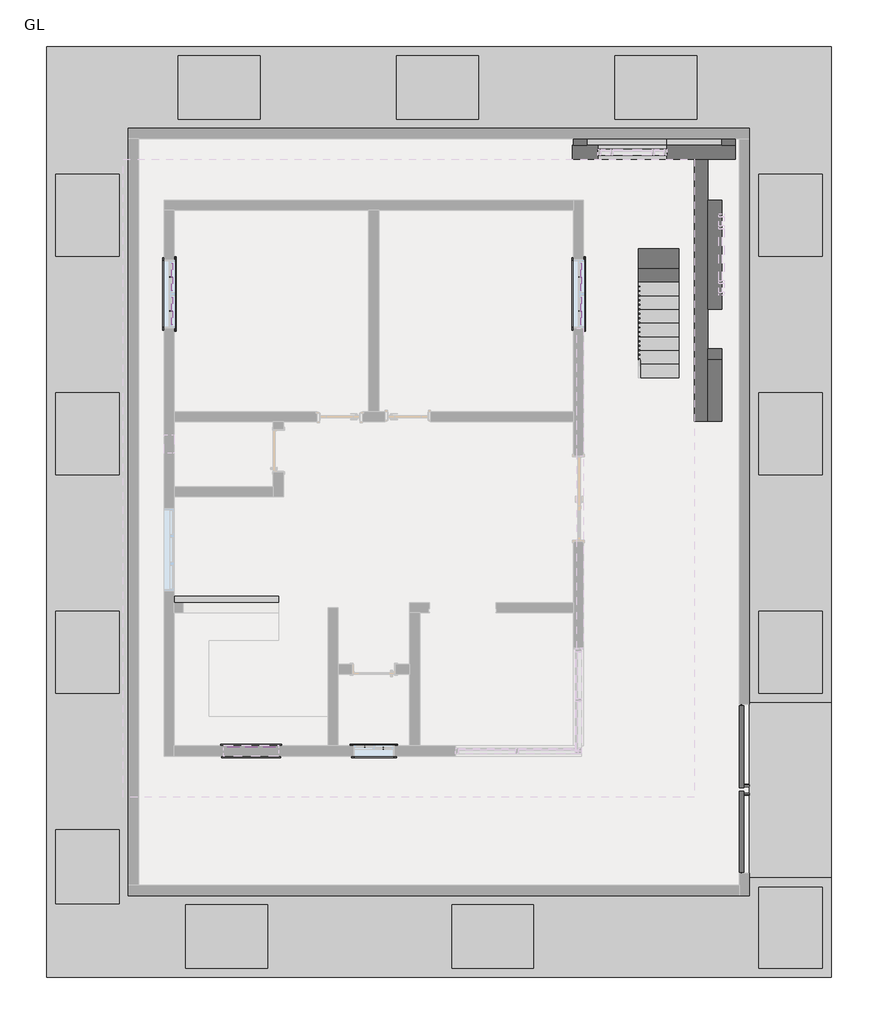
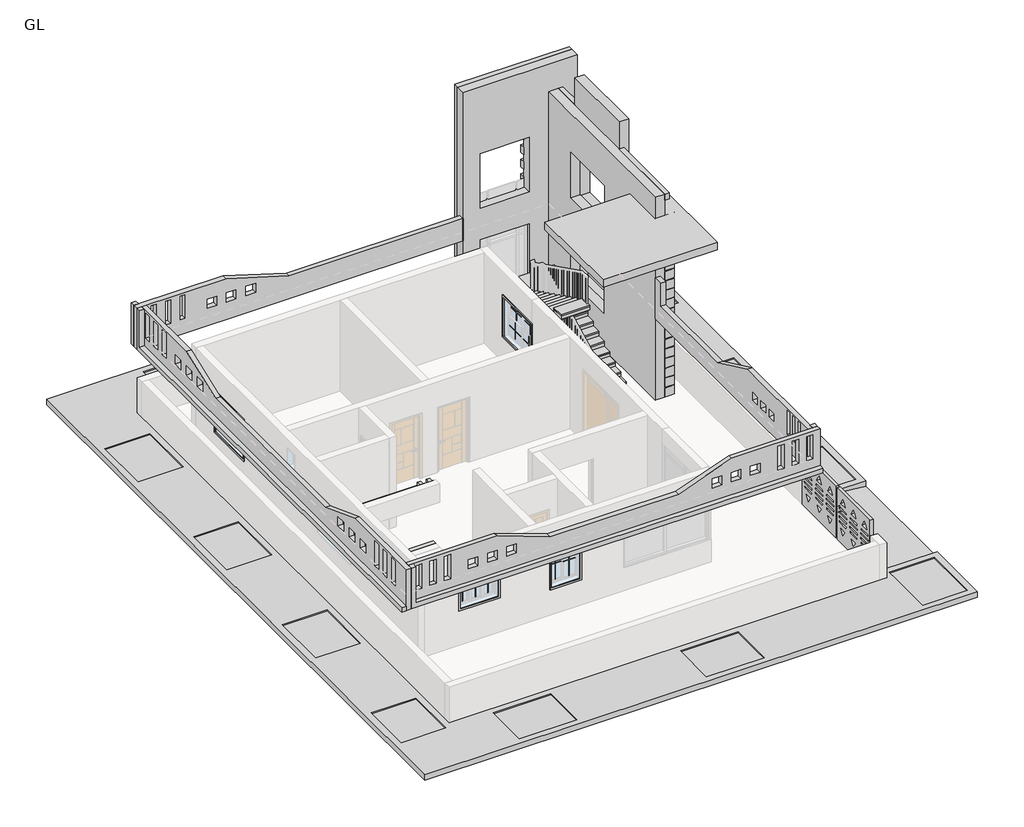
# One storey, part 4 of 4: 27 proxies, 1 stair flight.
"""IFC4 building model written with IfcOpenShell, lengths in millimetres."""

from ifc_helpers import new_model, si_unit, frame, origin, origin_with_axes, place, context, project, spatial, polyline, outline, extrude, faceted_brep, transform, mapped, element, save
from components import generic_models_477b0933, generic_models_1_generic_models_1_d084bfd0, generic_models_2_generic_models_2_55b91b29, generic_models_3_generic_models_3_9cf6d621, muntin_pattern_2x2_muntin_pattern_2x2_bf2d4cb0, muntin_pattern_2x2_muntin_pattern_2x2_60a90d43, muntin_pattern_2x2_muntin_pattern_2x2_daa3f335, muntin_pattern_2x2_muntin_pattern_2x2_453f50af, muntin_pattern_2x2_muntin_pattern_2x2_e8cdcc2d, ramp_ramp_f62ef563, trim_window_exterior_flat_with_sill_5d4eb4de, trim_window_exterior_flat_with_sill_e4b28ec3, trim_window_exterior_flat_with_sill_c4e67c73, trim_window_interior_flat_picture_frame_e325e1d2, trim_window_interior_flat_picture_frame_39ff4276, trim_window_interior_flat_picture_frame_cf1733af, front_elevation_front_elevation_9f25110b

model = new_model("IFC4")

# Units and contexts
model_context = context("Model", 3, world=origin())
ifc_project = project(units=[si_unit("LENGTHUNIT", "METRE", prefix="MILLI")], contexts=[model_context])

# Site, building, storey
site = spatial("IfcSite", under=ifc_project)
building = spatial("IfcBuilding", under=site)
storey = spatial("IfcBuildingStorey", under=building, Name="GL", Elevation=0.0)

# Proxies
placement = place(None, origin())
generic_models_shape = generic_models_477b0933(model_context)
element("IfcBuildingElementProxy", 1, Name="Generic Models", at=placement, inside=storey, context=model_context, shape_type="MappedRepresentation", body=[
    mapped(generic_models_shape, transform((1266.4722402, -2408.2657199, 0.0), x_axis=(0.0, 1.0, 0.0), y_axis=(-1.0, 0.0, 0.0), z_axis=(0.0, 0.0, 1.0))),
])
generic_models_1_generic_models_1_shape = generic_models_1_generic_models_1_d084bfd0(model_context)
element("IfcBuildingElementProxy", 2, Name="Generic Models 1 : Generic Models 1", ObjectType="Generic Models 1 : Generic Models 1", at=placement, inside=storey, context=model_context, shape_type="MappedRepresentation", body=[
    mapped(generic_models_1_generic_models_1_shape, transform((0.0, 0.0, 0.0), x_axis=(1.0, 0.0, 0.0), y_axis=(0.0, 1.0, 0.0), z_axis=(0.0, 0.0, 1.0))),
])
generic_models_2_generic_models_2_shape = generic_models_2_generic_models_2_55b91b29(model_context)
element("IfcBuildingElementProxy", 3, Name="Generic Models 2 : Generic Models 2", ObjectType="Generic Models 2 : Generic Models 2", at=placement, inside=storey, context=model_context, shape_type="MappedRepresentation", body=[
    mapped(generic_models_2_generic_models_2_shape, transform((0.0, 0.0, 0.0), x_axis=(1.0, 0.0, 0.0), y_axis=(0.0, 1.0, 0.0), z_axis=(0.0, 0.0, 1.0))),
])
generic_models_3_generic_models_3_shape = generic_models_3_generic_models_3_9cf6d621(model_context)
element("IfcBuildingElementProxy", 4, Name="Generic Models 3 : Generic Models 3", ObjectType="Generic Models 3 : Generic Models 3", at=placement, inside=storey, context=model_context, shape_type="MappedRepresentation", body=[
    mapped(generic_models_3_generic_models_3_shape, transform((0.0, 0.0, 0.0), x_axis=(1.0, 0.0, 0.0), y_axis=(0.0, 1.0, 0.0), z_axis=(0.0, 0.0, 1.0))),
])
muntin_pattern_2x2_muntin_pattern_2x2_shape = muntin_pattern_2x2_muntin_pattern_2x2_bf2d4cb0(model_context)
element("IfcBuildingElementProxy", 5, Name="Muntin Pattern_2x2 : Muntin Pattern_2x2", ObjectType="Muntin Pattern_2x2 : Muntin Pattern_2x2", at=placement, inside=storey, context=model_context, shape_type="MappedRepresentation", body=[
    mapped(muntin_pattern_2x2_muntin_pattern_2x2_shape, transform((-11392.2527598, 8590.7280301, 1597.025), x_axis=(0.0, -1.0, 0.0), y_axis=(1.0, 0.0, 0.0), z_axis=(0.0, 0.0, 1.0))),
])
element("IfcBuildingElementProxy", 6, Name="Muntin Pattern_2x2 : Muntin Pattern_2x2", ObjectType="Muntin Pattern_2x2 : Muntin Pattern_2x2", at=placement, inside=storey, context=model_context, shape_type="MappedRepresentation", body=[
    mapped(muntin_pattern_2x2_muntin_pattern_2x2_shape, transform((-11436.7027598, 8590.7280301, 990.6), x_axis=(0.0, -1.0, 0.0), y_axis=(1.0, 0.0, 0.0), z_axis=(0.0, 0.0, 1.0))),
])
element("IfcBuildingElementProxy", 7, Name="Muntin Pattern_2x2 : Muntin Pattern_2x2", ObjectType="Muntin Pattern_2x2 : Muntin Pattern_2x2", at=placement, inside=storey, context=model_context, shape_type="MappedRepresentation", body=[
    mapped(muntin_pattern_2x2_muntin_pattern_2x2_shape, transform((-2248.2527598, 8590.7280301, 1597.025), x_axis=(0.0, -1.0, 0.0), y_axis=(1.0, 0.0, 0.0), z_axis=(0.0, 0.0, 1.0))),
])
element("IfcBuildingElementProxy", 8, Name="Muntin Pattern_2x2 : Muntin Pattern_2x2", ObjectType="Muntin Pattern_2x2 : Muntin Pattern_2x2", at=placement, inside=storey, context=model_context, shape_type="MappedRepresentation", body=[
    mapped(muntin_pattern_2x2_muntin_pattern_2x2_shape, transform((-2292.7027598, 8590.7280301, 990.6), x_axis=(0.0, -1.0, 0.0), y_axis=(1.0, 0.0, 0.0), z_axis=(0.0, 0.0, 1.0))),
])
muntin_pattern_2x2_muntin_pattern_2x2_2_shape = muntin_pattern_2x2_muntin_pattern_2x2_60a90d43(model_context)
element("IfcBuildingElementProxy", 9, Name="Muntin Pattern_2x2 : Muntin Pattern_2x2", ObjectType="Muntin Pattern_2x2 : Muntin Pattern_2x2", at=placement, inside=storey, context=model_context, shape_type="MappedRepresentation", body=[
    mapped(muntin_pattern_2x2_muntin_pattern_2x2_2_shape, transform((-11392.2527598, 9351.1405301, 1597.025), x_axis=(0.0, 1.0, 0.0), y_axis=(-1.0, 0.0, 0.0), z_axis=(0.0, 0.0, 1.0))),
])
element("IfcBuildingElementProxy", 10, Name="Muntin Pattern_2x2 : Muntin Pattern_2x2", ObjectType="Muntin Pattern_2x2 : Muntin Pattern_2x2", at=placement, inside=storey, context=model_context, shape_type="MappedRepresentation", body=[
    mapped(muntin_pattern_2x2_muntin_pattern_2x2_2_shape, transform((-11436.7027598, 9351.1405301, 990.6), x_axis=(0.0, 1.0, 0.0), y_axis=(-1.0, 0.0, 0.0), z_axis=(0.0, 0.0, 1.0))),
])
element("IfcBuildingElementProxy", 11, Name="Muntin Pattern_2x2 : Muntin Pattern_2x2", ObjectType="Muntin Pattern_2x2 : Muntin Pattern_2x2", at=placement, inside=storey, context=model_context, shape_type="MappedRepresentation", body=[
    mapped(muntin_pattern_2x2_muntin_pattern_2x2_2_shape, transform((-2248.2527598, 9351.1405301, 1597.025), x_axis=(0.0, 1.0, 0.0), y_axis=(-1.0, 0.0, 0.0), z_axis=(0.0, 0.0, 1.0))),
])
element("IfcBuildingElementProxy", 12, Name="Muntin Pattern_2x2 : Muntin Pattern_2x2", ObjectType="Muntin Pattern_2x2 : Muntin Pattern_2x2", at=placement, inside=storey, context=model_context, shape_type="MappedRepresentation", body=[
    mapped(muntin_pattern_2x2_muntin_pattern_2x2_2_shape, transform((-2292.7027598, 9351.1405301, 990.6), x_axis=(0.0, 1.0, 0.0), y_axis=(-1.0, 0.0, 0.0), z_axis=(0.0, 0.0, 1.0))),
])
muntin_pattern_2x2_muntin_pattern_2x2_3_shape = muntin_pattern_2x2_muntin_pattern_2x2_daa3f335(model_context)
element("IfcBuildingElementProxy", 13, Name="Muntin Pattern_2x2 : Muntin Pattern_2x2", ObjectType="Muntin Pattern_2x2 : Muntin Pattern_2x2", at=placement, inside=storey, context=model_context, shape_type="MappedRepresentation", body=[
    mapped(muntin_pattern_2x2_muntin_pattern_2x2_3_shape, transform((-6691.6652598, -1179.5407199, 996.95), x_axis=(1.0, 0.0, 0.0), y_axis=(0.0, 1.0, 0.0), z_axis=(0.0, 0.0, 1.0))),
])
element("IfcBuildingElementProxy", 14, Name="Muntin Pattern_2x2 : Muntin Pattern_2x2", ObjectType="Muntin Pattern_2x2 : Muntin Pattern_2x2", at=placement, inside=storey, context=model_context, shape_type="MappedRepresentation", body=[
    mapped(muntin_pattern_2x2_muntin_pattern_2x2_3_shape, transform((-7107.5902598, -1135.0907199, 996.95), x_axis=(1.0, 0.0, 0.0), y_axis=(0.0, 1.0, 0.0), z_axis=(0.0, 0.0, 1.0))),
])
muntin_pattern_2x2_muntin_pattern_2x2_4_shape = muntin_pattern_2x2_muntin_pattern_2x2_453f50af(model_context)
element("IfcBuildingElementProxy", 15, Name="Muntin Pattern_2x2 : Muntin Pattern_2x2", ObjectType="Muntin Pattern_2x2 : Muntin Pattern_2x2", at=placement, inside=storey, context=model_context, shape_type="MappedRepresentation", body=[
    mapped(muntin_pattern_2x2_muntin_pattern_2x2_4_shape, transform((-10047.1110931, -1135.0907199, 1289.05), x_axis=(1.0, 0.0, 0.0), y_axis=(0.0, 1.0, 0.0), z_axis=(0.0, 0.0, 1.0))),
])
muntin_pattern_2x2_muntin_pattern_2x2_5_shape = muntin_pattern_2x2_muntin_pattern_2x2_e8cdcc2d(model_context)
element("IfcBuildingElementProxy", 16, Name="Muntin Pattern_2x2 : Muntin Pattern_2x2", ObjectType="Muntin Pattern_2x2 : Muntin Pattern_2x2", at=placement, inside=storey, context=model_context, shape_type="MappedRepresentation", body=[
    mapped(muntin_pattern_2x2_muntin_pattern_2x2_5_shape, transform((-9238.5444264, -1135.0907199, 1289.05), x_axis=(-1.0, 0.0, 0.0), y_axis=(0.0, -1.0, 0.0), z_axis=(0.0, 0.0, 1.0))),
])
element("IfcBuildingElementProxy", 17, Name="Muntin Pattern_2x2 : Muntin Pattern_2x2", ObjectType="Muntin Pattern_2x2 : Muntin Pattern_2x2", at=placement, inside=storey, context=model_context, shape_type="MappedRepresentation", body=[
    mapped(muntin_pattern_2x2_muntin_pattern_2x2_5_shape, transform((-9642.8277598, -1135.0907199, 1289.05), x_axis=(-1.0, 0.0, 0.0), y_axis=(0.0, -1.0, 0.0), z_axis=(0.0, 0.0, 1.0))),
])
ramp_ramp_shape = ramp_ramp_f62ef563(model_context)
element("IfcBuildingElementProxy", 18, Name="RAMP : RAMP", ObjectType="RAMP : RAMP", at=placement, inside=storey, context=model_context, shape_type="MappedRepresentation", body=[
    mapped(ramp_ramp_shape, transform((0.0, 0.0, 0.0), x_axis=(1.0, 0.0, 0.0), y_axis=(0.0, 1.0, 0.0), z_axis=(0.0, 0.0, 1.0))),
])
trim_window_exterior_flat_with_sill_shape = trim_window_exterior_flat_with_sill_5d4eb4de(model_context)
element("IfcBuildingElementProxy", 19, Name="Trim-Window-Exterior-Flat : with Sill", ObjectType="Trim-Window-Exterior-Flat : with Sill", at=placement, inside=storey, context=model_context, shape_type="MappedRepresentation", body=[
    mapped(trim_window_exterior_flat_with_sill_shape, transform((-11357.3277598, 8970.9342801, 2235.2), x_axis=(0.0, 1.0, 0.0), y_axis=(0.0, 0.0, 1.0), z_axis=(1.0, 0.0, 0.0))),
])
element("IfcBuildingElementProxy", 20, Name="Trim-Window-Exterior-Flat : with Sill", ObjectType="Trim-Window-Exterior-Flat : with Sill", at=placement, inside=storey, context=model_context, shape_type="MappedRepresentation", body=[
    mapped(trim_window_exterior_flat_with_sill_shape, transform((-2213.3277598, 8970.9342801, 2235.2), x_axis=(0.0, 1.0, 0.0), y_axis=(0.0, 0.0, 1.0), z_axis=(1.0, 0.0, 0.0))),
])
trim_window_exterior_flat_with_sill_2_shape = trim_window_exterior_flat_with_sill_e4b28ec3(model_context)
element("IfcBuildingElementProxy", 21, Name="Trim-Window-Exterior-Flat : with Sill", ObjectType="Trim-Window-Exterior-Flat : with Sill", at=placement, inside=storey, context=model_context, shape_type="MappedRepresentation", body=[
    mapped(trim_window_exterior_flat_with_sill_2_shape, transform((-6899.6277598, -1125.5657199, 2133.6), x_axis=(-1.0, 0.0, 0.0), y_axis=(0.0, 0.0, 1.0), z_axis=(0.0, 1.0, 0.0))),
])
trim_window_exterior_flat_with_sill_3_shape = trim_window_exterior_flat_with_sill_c4e67c73(model_context)
element("IfcBuildingElementProxy", 22, Name="Trim-Window-Exterior-Flat : with Sill", ObjectType="Trim-Window-Exterior-Flat : with Sill", at=placement, inside=storey, context=model_context, shape_type="MappedRepresentation", body=[
    mapped(trim_window_exterior_flat_with_sill_3_shape, transform((-9642.8277598, -1125.5657199, 2133.6), x_axis=(-1.0, 0.0, 0.0), y_axis=(0.0, 0.0, 1.0), z_axis=(0.0, 1.0, 0.0))),
])
trim_window_interior_flat_picture_frame_shape = trim_window_interior_flat_picture_frame_e325e1d2(model_context)
element("IfcBuildingElementProxy", 23, Name="Trim-Window-Interior-Flat : Picture Frame", ObjectType="Trim-Window-Interior-Flat : Picture Frame", at=placement, inside=storey, context=model_context, shape_type="MappedRepresentation", body=[
    mapped(trim_window_interior_flat_picture_frame_shape, transform((-11585.9277598, 8970.9342801, 2235.2), x_axis=(0.0, -1.0, 0.0), y_axis=(0.0, 0.0, 1.0), z_axis=(-1.0, 0.0, 0.0))),
])
element("IfcBuildingElementProxy", 24, Name="Trim-Window-Interior-Flat : Picture Frame", ObjectType="Trim-Window-Interior-Flat : Picture Frame", at=placement, inside=storey, context=model_context, shape_type="MappedRepresentation", body=[
    mapped(trim_window_interior_flat_picture_frame_shape, transform((-2441.9277598, 8970.9342801, 2235.2), x_axis=(0.0, -1.0, 0.0), y_axis=(0.0, 0.0, 1.0), z_axis=(-1.0, 0.0, 0.0))),
])
trim_window_interior_flat_picture_frame_2_shape = trim_window_interior_flat_picture_frame_39ff4276(model_context)
element("IfcBuildingElementProxy", 25, Name="Trim-Window-Interior-Flat : Picture Frame", ObjectType="Trim-Window-Interior-Flat : Picture Frame", at=placement, inside=storey, context=model_context, shape_type="MappedRepresentation", body=[
    mapped(trim_window_interior_flat_picture_frame_2_shape, transform((-6899.6277598, -1354.1657199, 2133.6), x_axis=(1.0, 0.0, 0.0), y_axis=(0.0, 0.0, 1.0), z_axis=(0.0, -1.0, 0.0))),
])
trim_window_interior_flat_picture_frame_3_shape = trim_window_interior_flat_picture_frame_cf1733af(model_context)
element("IfcBuildingElementProxy", 26, Name="Trim-Window-Interior-Flat : Picture Frame", ObjectType="Trim-Window-Interior-Flat : Picture Frame", at=placement, inside=storey, context=model_context, shape_type="MappedRepresentation", body=[
    mapped(trim_window_interior_flat_picture_frame_3_shape, transform((-9642.8277598, -1354.1657199, 2133.6), x_axis=(1.0, 0.0, 0.0), y_axis=(0.0, 0.0, 1.0), z_axis=(0.0, -1.0, 0.0))),
])
front_elevation_front_elevation_shape = front_elevation_front_elevation_9f25110b(model_context)
element("IfcBuildingElementProxy", 27, Name="front elevation : front elevation", ObjectType="front elevation : front elevation", at=placement, inside=storey, context=model_context, shape_type="MappedRepresentation", body=[
    mapped(front_elevation_front_elevation_shape, transform((0.0, 0.0, 0.0), x_axis=(1.0, 0.0, 0.0), y_axis=(0.0, 1.0, 0.0), z_axis=(0.0, 0.0, 1.0))),
])

# Stair flight
element("IfcStairFlight", 28, ObjectType="3/4\" Nosing 6 1/2\" Depth", at=placement, inside=storey, context=model_context, shape_type="SolidModel", body=[
    faceted_brep([(-994.1277598, 7415.1842801, 101.6), (-994.1277598, 7110.3842801, 101.6), (-79.7277598, 7110.3842801, 101.6), (-79.7277598, 7415.1842801, 101.6), (-994.1277598, 7415.1842801, 0.0), (-994.1277598, 7110.3842801, 0.0), (-79.7277598, 7110.3842801, 0.0), (-79.7277598, 7415.1842801, 0.0), (-994.1277598, 7719.9842801, 254.0), (-994.1277598, 7415.1842801, 254.0), (-79.7277598, 7415.1842801, 254.0), (-79.7277598, 7719.9842801, 254.0), (-994.1277598, 7719.9842801, 69.4125885), (-994.1277598, 7581.1591032, 0.0), (-79.7277598, 7581.1591032, 0.0), (-79.7277598, 7719.9842801, 69.4125885), (-994.1277598, 8024.7842801, 406.4), (-994.1277598, 7719.9842801, 406.4), (-79.7277598, 7719.9842801, 406.4), (-79.7277598, 8024.7842801, 406.4), (-994.1277598, 8024.7842801, 221.8125885), (-79.7277598, 8024.7842801, 221.8125885), (-994.1277598, 8329.5842801, 558.8), (-994.1277598, 8024.7842801, 558.8), (-79.7277598, 8024.7842801, 558.8), (-79.7277598, 8329.5842801, 558.8), (-994.1277598, 8329.5842801, 374.2125885), (-79.7277598, 8329.5842801, 374.2125885), (-994.1277598, 8634.3842801, 711.2), (-994.1277598, 8329.5842801, 711.2), (-79.7277598, 8329.5842801, 711.2), (-79.7277598, 8634.3842801, 711.2), (-994.1277598, 8634.3842801, 526.6125885), (-79.7277598, 8634.3842801, 526.6125885), (-994.1277598, 8939.1842801, 863.6), (-994.1277598, 8634.3842801, 863.6), (-79.7277598, 8634.3842801, 863.6), (-79.7277598, 8939.1842801, 863.6), (-994.1277598, 8939.1842801, 679.0125885), (-79.7277598, 8939.1842801, 679.0125885), (-994.1277598, 9243.9842801, 1016.0), (-994.1277598, 8939.1842801, 1016.0), (-79.7277598, 8939.1842801, 1016.0), (-79.7277598, 9243.9842801, 1016.0), (-994.1277598, 9243.9842801, 831.4125885), (-79.7277598, 9243.9842801, 831.4125885), (-994.1277598, 9548.7842801, 1168.4), (-994.1277598, 9243.9842801, 1168.4), (-79.7277598, 9243.9842801, 1168.4), (-79.7277598, 9548.7842801, 1168.4), (-994.1277598, 9548.7842801, 983.8125885), (-79.7277598, 9548.7842801, 983.8125885), (-994.1277598, 9853.5842801, 1320.8), (-994.1277598, 9548.7842801, 1320.8), (-79.7277598, 9548.7842801, 1320.8), (-79.7277598, 9853.5842801, 1320.8), (-994.1277598, 9853.5842801, 1136.2125885), (-79.7277598, 9853.5842801, 1136.2125885), (-994.1277598, 9853.5842801, 1473.2), (-79.7277598, 9853.5842801, 1473.2), (-79.7277598, 10158.3842801, 1473.2), (-994.1277598, 10158.3842801, 1473.2), (-994.1277598, 10152.0342801, 1473.2), (-994.1277598, 10152.0342801, 1460.5), (-994.1277598, 10502.1591032, 1460.5), (-79.7277598, 10158.3842801, 1288.6125885), (-1298.9277598, 10145.6842801, 1625.6), (-1298.9277598, 10152.0342801, 1625.6), (-994.1277598, 10152.0342801, 1625.6), (-994.1277598, 10158.3842801, 1625.6), (-79.7277598, 10158.3842801, 1625.6), (-79.7277598, 10502.1591032, 1625.6), (-79.7277598, 11066.4342801, 1625.6), (-2213.3277598, 11066.4342801, 1625.6), (-2213.3277598, 10145.6842801, 1625.6), (-1298.9277598, 10145.6842801, 1460.5), (-1298.9277598, 10152.0342801, 1460.5), (-79.7277598, 10502.1591032, 1460.5), (-79.7277598, 11066.4342801, 1460.5), (-2213.3277598, 11066.4342801, 1460.5), (-2213.3277598, 10145.6842801, 1460.5), (-1298.9277598, 10145.6842801, 1778.0), (-2213.3277598, 10145.6842801, 1778.0), (-2213.3277598, 10106.7094571, 1778.0), (-2213.3277598, 9840.8842801, 1778.0), (-1298.9277598, 9840.8842801, 1778.0), (-1298.9277598, 10106.7094571, 1778.0), (-1298.9277598, 9840.8842801, 1593.4125885), (-1298.9277598, 10106.7094571, 1460.5), (-2213.3277598, 10106.7094571, 1460.5), (-2213.3277598, 9840.8842801, 1593.4125885), (-1298.9277598, 9536.0842801, 1930.4), (-1298.9277598, 9840.8842801, 1930.4), (-2213.3277598, 9840.8842801, 1930.4), (-2213.3277598, 9536.0842801, 1930.4), (-1298.9277598, 9536.0842801, 1745.8125885), (-2213.3277598, 9536.0842801, 1745.8125885), (-1298.9277598, 9231.2842801, 2082.8), (-1298.9277598, 9536.0842801, 2082.8), (-2213.3277598, 9536.0842801, 2082.8), (-2213.3277598, 9231.2842801, 2082.8), (-1298.9277598, 9231.2842801, 1898.2125885), (-2213.3277598, 9231.2842801, 1898.2125885), (-1298.9277598, 8926.4842801, 2235.2), (-1298.9277598, 9231.2842801, 2235.2), (-2213.3277598, 9231.2842801, 2235.2), (-2213.3277598, 8926.4842801, 2235.2), (-1298.9277598, 8926.4842801, 2050.6125885), (-2213.3277598, 8926.4842801, 2050.6125885), (-1298.9277598, 8621.6842801, 2387.6), (-1298.9277598, 8926.4842801, 2387.6), (-2213.3277598, 8926.4842801, 2387.6), (-2213.3277598, 8621.6842801, 2387.6), (-1298.9277598, 8621.6842801, 2203.0125885), (-2213.3277598, 8621.6842801, 2203.0125885), (-1298.9277598, 8316.8842801, 2540.0), (-1298.9277598, 8621.6842801, 2540.0), (-2213.3277598, 8621.6842801, 2540.0), (-2213.3277598, 8316.8842801, 2540.0), (-1298.9277598, 8316.8842801, 2355.4125885), (-2213.3277598, 8316.8842801, 2355.4125885), (-1298.9277598, 8012.0842801, 2692.4), (-1298.9277598, 8316.8842801, 2692.4), (-2213.3277598, 8316.8842801, 2692.4), (-2213.3277598, 8012.0842801, 2692.4), (-1298.9277598, 8012.0842801, 2507.8125885), (-2213.3277598, 8012.0842801, 2507.8125885), (-1298.9277598, 7707.2842801, 2844.8), (-1298.9277598, 8012.0842801, 2844.8), (-2213.3277598, 8012.0842801, 2844.8), (-2213.3277598, 7707.2842801, 2844.8), (-1298.9277598, 7707.2842801, 2660.2125885), (-2213.3277598, 7707.2842801, 2660.2125885), (-1298.9277598, 7402.4842801, 2997.2), (-1298.9277598, 7707.2842801, 2997.2), (-2213.3277598, 7707.2842801, 2997.2), (-2213.3277598, 7402.4842801, 2997.2), (-1298.9277598, 7402.4842801, 2812.6125885), (-2213.3277598, 7402.4842801, 2812.6125885), (-1298.9277598, 7402.4842801, 3149.6), (-2213.3277598, 7402.4842801, 3149.6), (-2213.3277598, 7002.4342801, 3149.6), (-1298.9277598, 7002.4342801, 3149.6), (-1298.9277598, 7002.4342801, 3048.0), (-1298.9277598, 7104.0342801, 3048.0), (-1298.9277598, 7104.0342801, 2961.8375885), (-2213.3277598, 7104.0342801, 2961.8375885), (-2213.3277598, 7104.0342801, 3048.0), (-2213.3277598, 7002.4342801, 3048.0)], [[[0, 1, 2, 3]], [[1, 0, 4, 5]], [[2, 1, 5, 6]], [[3, 2, 6, 7]], [[8, 9, 10, 11]], [[4, 0, 9, 8, 12, 13]], [[0, 3, 10, 9]], [[3, 7, 14, 15, 11, 10]], [[16, 17, 18, 19]], [[17, 16, 20, 12, 8]], [[8, 11, 18, 17]], [[19, 18, 11, 15, 21]], [[22, 23, 24, 25]], [[23, 22, 26, 20, 16]], [[16, 19, 24, 23]], [[25, 24, 19, 21, 27]], [[28, 29, 30, 31]], [[29, 28, 32, 26, 22]], [[22, 25, 30, 29]], [[31, 30, 25, 27, 33]], [[34, 35, 36, 37]], [[35, 34, 38, 32, 28]], [[28, 31, 36, 35]], [[37, 36, 31, 33, 39]], [[40, 41, 42, 43]], [[41, 40, 44, 38, 34]], [[34, 37, 42, 41]], [[43, 42, 37, 39, 45]], [[46, 47, 48, 49]], [[47, 46, 50, 44, 40]], [[40, 43, 48, 47]], [[49, 48, 43, 45, 51]], [[52, 53, 54, 55]], [[53, 52, 56, 50, 46]], [[46, 49, 54, 53]], [[55, 54, 49, 51, 57]], [[58, 59, 60, 61, 62]], [[58, 62, 63, 64, 56, 52]], [[52, 55, 59, 58]], [[60, 59, 55, 57, 65]], [[66, 67, 68, 69, 70, 71, 72, 73, 74]], [[67, 66, 75, 76]], [[68, 67, 76, 63, 62]], [[62, 61, 69, 68]], [[61, 60, 70, 69]], [[70, 60, 65, 77, 78, 72, 71]], [[73, 72, 78, 79]], [[74, 73, 79, 80]], [[81, 82, 83, 84, 85, 86]], [[66, 81, 86, 85, 87, 88, 75]], [[66, 74, 82, 81]], [[82, 74, 80, 89, 90, 84, 83]], [[91, 92, 93, 94]], [[92, 91, 95, 87, 85]], [[85, 84, 93, 92]], [[94, 93, 84, 90, 96]], [[97, 98, 99, 100]], [[98, 97, 101, 95, 91]], [[91, 94, 99, 98]], [[100, 99, 94, 96, 102]], [[103, 104, 105, 106]], [[104, 103, 107, 101, 97]], [[97, 100, 105, 104]], [[106, 105, 100, 102, 108]], [[109, 110, 111, 112]], [[110, 109, 113, 107, 103]], [[103, 106, 111, 110]], [[112, 111, 106, 108, 114]], [[115, 116, 117, 118]], [[116, 115, 119, 113, 109]], [[109, 112, 117, 116]], [[118, 117, 112, 114, 120]], [[121, 122, 123, 124]], [[122, 121, 125, 119, 115]], [[115, 118, 123, 122]], [[124, 123, 118, 120, 126]], [[127, 128, 129, 130]], [[128, 127, 131, 125, 121]], [[121, 124, 129, 128]], [[130, 129, 124, 126, 132]], [[133, 134, 135, 136]], [[134, 133, 137, 131, 127]], [[127, 130, 135, 134]], [[136, 135, 130, 132, 138]], [[139, 140, 141, 142]], [[139, 142, 143, 144, 145, 137, 133]], [[133, 136, 140, 139]], [[141, 140, 136, 138, 146, 147, 148]], [[146, 145, 144, 147]], [[5, 4, 13, 14, 7, 6]], [[64, 77, 65, 57, 51, 45, 39, 33, 27, 21, 15, 14, 13, 12, 20, 26, 32, 38, 44, 50, 56]], [[77, 64, 63, 76, 75, 88, 89, 80, 79, 78]], [[89, 88, 87, 95, 101, 107, 113, 119, 125, 131, 137, 145, 146, 138, 132, 126, 120, 114, 108, 102, 96, 90]], [[148, 147, 144, 143]], [[148, 143, 142, 141]]]),
    extrude(outline(polyline([(-994.1277598, 7408.8342801), (-79.7277598, 7408.8342801), (-79.7277598, 7104.0342801), (-994.1277598, 7104.0342801), (-994.1277598, 7408.8342801)])), frame((0.0, 0.0, 101.6), z_axis=(0.0, 0.0, 1.0), x_axis=(1.0, 0.0, 0.0)), (0.0, 0.0, 1.0), 50.8),
    extrude(outline(polyline([(-79.7277598, 7110.3842801), (-79.7277598, 7104.0342801), (-994.1277598, 7104.0342801), (-994.1277598, 7110.3842801), (-79.7277598, 7110.3842801)])), origin_with_axes(), (0.0, 0.0, 1.0), 101.6),
    extrude(outline(polyline([(-79.7277598, 7415.1842801), (-79.7277598, 7408.8342801), (-994.1277598, 7408.8342801), (-994.1277598, 7415.1842801), (-79.7277598, 7415.1842801)])), frame((0.0, 0.0, 101.6), z_axis=(0.0, 0.0, 1.0), x_axis=(1.0, 0.0, 0.0)), (0.0, 0.0, 1.0), 152.4),
    extrude(outline(polyline([(-994.1277598, 7713.6342801), (-79.7277598, 7713.6342801), (-79.7277598, 7408.8342801), (-994.1277598, 7408.8342801), (-994.1277598, 7713.6342801)])), frame((0.0, 0.0, 254.0), z_axis=(0.0, 0.0, 1.0), x_axis=(1.0, 0.0, 0.0)), (0.0, 0.0, 1.0), 50.8),
    extrude(outline(polyline([(-79.7277598, 7719.9842801), (-79.7277598, 7713.6342801), (-994.1277598, 7713.6342801), (-994.1277598, 7719.9842801), (-79.7277598, 7719.9842801)])), frame((0.0, 0.0, 254.0), z_axis=(0.0, 0.0, 1.0), x_axis=(1.0, 0.0, 0.0)), (0.0, 0.0, 1.0), 152.4),
    extrude(outline(polyline([(-994.1277598, 8018.4342801), (-79.7277598, 8018.4342801), (-79.7277598, 7713.6342801), (-994.1277598, 7713.6342801), (-994.1277598, 8018.4342801)])), frame((0.0, 0.0, 406.4), z_axis=(0.0, 0.0, 1.0), x_axis=(1.0, 0.0, 0.0)), (0.0, 0.0, 1.0), 50.8),
    extrude(outline(polyline([(-79.7277598, 8024.7842801), (-79.7277598, 8018.4342801), (-994.1277598, 8018.4342801), (-994.1277598, 8024.7842801), (-79.7277598, 8024.7842801)])), frame((0.0, 0.0, 406.4), z_axis=(0.0, 0.0, 1.0), x_axis=(1.0, 0.0, 0.0)), (0.0, 0.0, 1.0), 152.4),
    extrude(outline(polyline([(-994.1277598, 8323.2342801), (-79.7277598, 8323.2342801), (-79.7277598, 8018.4342801), (-994.1277598, 8018.4342801), (-994.1277598, 8323.2342801)])), frame((0.0, 0.0, 558.8), z_axis=(0.0, 0.0, 1.0), x_axis=(1.0, 0.0, 0.0)), (0.0, 0.0, 1.0), 50.8),
    extrude(outline(polyline([(-79.7277598, 8329.5842801), (-79.7277598, 8323.2342801), (-994.1277598, 8323.2342801), (-994.1277598, 8329.5842801), (-79.7277598, 8329.5842801)])), frame((0.0, 0.0, 558.8), z_axis=(0.0, 0.0, 1.0), x_axis=(1.0, 0.0, 0.0)), (0.0, 0.0, 1.0), 152.4),
    extrude(outline(polyline([(-994.1277598, 8628.0342801), (-79.7277598, 8628.0342801), (-79.7277598, 8323.2342801), (-994.1277598, 8323.2342801), (-994.1277598, 8628.0342801)])), frame((0.0, 0.0, 711.2), z_axis=(0.0, 0.0, 1.0), x_axis=(1.0, 0.0, 0.0)), (0.0, 0.0, 1.0), 50.8),
    extrude(outline(polyline([(-79.7277598, 8634.3842801), (-79.7277598, 8628.0342801), (-994.1277598, 8628.0342801), (-994.1277598, 8634.3842801), (-79.7277598, 8634.3842801)])), frame((0.0, 0.0, 711.2), z_axis=(0.0, 0.0, 1.0), x_axis=(1.0, 0.0, 0.0)), (0.0, 0.0, 1.0), 152.4),
    extrude(outline(polyline([(-994.1277598, 8932.8342801), (-79.7277598, 8932.8342801), (-79.7277598, 8628.0342801), (-994.1277598, 8628.0342801), (-994.1277598, 8932.8342801)])), frame((0.0, 0.0, 863.6), z_axis=(0.0, 0.0, 1.0), x_axis=(1.0, 0.0, 0.0)), (0.0, 0.0, 1.0), 50.8),
    extrude(outline(polyline([(-79.7277598, 8939.1842801), (-79.7277598, 8932.8342801), (-994.1277598, 8932.8342801), (-994.1277598, 8939.1842801), (-79.7277598, 8939.1842801)])), frame((0.0, 0.0, 863.6), z_axis=(0.0, 0.0, 1.0), x_axis=(1.0, 0.0, 0.0)), (0.0, 0.0, 1.0), 152.4),
    extrude(outline(polyline([(-994.1277598, 9237.6342801), (-79.7277598, 9237.6342801), (-79.7277598, 8932.8342801), (-994.1277598, 8932.8342801), (-994.1277598, 9237.6342801)])), frame((0.0, 0.0, 1016.0), z_axis=(0.0, 0.0, 1.0), x_axis=(1.0, 0.0, 0.0)), (0.0, 0.0, 1.0), 50.8),
    extrude(outline(polyline([(-79.7277598, 9243.9842801), (-79.7277598, 9237.6342801), (-994.1277598, 9237.6342801), (-994.1277598, 9243.9842801), (-79.7277598, 9243.9842801)])), frame((0.0, 0.0, 1016.0), z_axis=(0.0, 0.0, 1.0), x_axis=(1.0, 0.0, 0.0)), (0.0, 0.0, 1.0), 152.4),
    extrude(outline(polyline([(-994.1277598, 9542.4342801), (-79.7277598, 9542.4342801), (-79.7277598, 9237.6342801), (-994.1277598, 9237.6342801), (-994.1277598, 9542.4342801)])), frame((0.0, 0.0, 1168.4), z_axis=(0.0, 0.0, 1.0), x_axis=(1.0, 0.0, 0.0)), (0.0, 0.0, 1.0), 50.8),
    extrude(outline(polyline([(-79.7277598, 9548.7842801), (-79.7277598, 9542.4342801), (-994.1277598, 9542.4342801), (-994.1277598, 9548.7842801), (-79.7277598, 9548.7842801)])), frame((0.0, 0.0, 1168.4), z_axis=(0.0, 0.0, 1.0), x_axis=(1.0, 0.0, 0.0)), (0.0, 0.0, 1.0), 152.4),
    extrude(outline(polyline([(-994.1277598, 9847.2342801), (-79.7277598, 9847.2342801), (-79.7277598, 9542.4342801), (-994.1277598, 9542.4342801), (-994.1277598, 9847.2342801)])), frame((0.0, 0.0, 1320.8), z_axis=(0.0, 0.0, 1.0), x_axis=(1.0, 0.0, 0.0)), (0.0, 0.0, 1.0), 50.8),
    extrude(outline(polyline([(-79.7277598, 9853.5842801), (-79.7277598, 9847.2342801), (-994.1277598, 9847.2342801), (-994.1277598, 9853.5842801), (-79.7277598, 9853.5842801)])), frame((0.0, 0.0, 1320.8), z_axis=(0.0, 0.0, 1.0), x_axis=(1.0, 0.0, 0.0)), (0.0, 0.0, 1.0), 152.4),
    extrude(outline(polyline([(-994.1277598, 10152.0342801), (-79.7277598, 10152.0342801), (-79.7277598, 9847.2342801), (-994.1277598, 9847.2342801), (-994.1277598, 10152.0342801)])), frame((0.0, 0.0, 1473.2), z_axis=(0.0, 0.0, 1.0), x_axis=(1.0, 0.0, 0.0)), (0.0, 0.0, 1.0), 50.8),
    extrude(outline(polyline([(-79.7277598, 10158.3842801), (-79.7277598, 10152.0342801), (-994.1277598, 10152.0342801), (-994.1277598, 10158.3842801), (-79.7277598, 10158.3842801)])), frame((0.0, 0.0, 1473.2), z_axis=(0.0, 0.0, 1.0), x_axis=(1.0, 0.0, 0.0)), (0.0, 0.0, 1.0), 152.4),
    extrude(outline(polyline([(-1298.9277598, 10152.0342801), (-2213.3277598, 10152.0342801), (-2213.3277598, 11066.4342801), (-79.7277598, 11066.4342801), (-79.7277598, 10152.0342801), (-994.1277598, 10152.0342801), (-1298.9277598, 10152.0342801)])), frame((0.0, 0.0, 1625.6), z_axis=(0.0, 0.0, 1.0), x_axis=(1.0, 0.0, 0.0)), (0.0, 0.0, 1.0), 50.8),
    extrude(outline(polyline([(-2213.3277598, 10145.6842801), (-2213.3277598, 10152.0342801), (-1298.9277598, 10152.0342801), (-1298.9277598, 10145.6842801), (-2213.3277598, 10145.6842801)])), frame((0.0, 0.0, 1625.6), z_axis=(0.0, 0.0, 1.0), x_axis=(1.0, 0.0, 0.0)), (0.0, 0.0, 1.0), 152.4),
    extrude(outline(polyline([(-1298.9277598, 9847.2342801), (-2213.3277598, 9847.2342801), (-2213.3277598, 10152.0342801), (-1298.9277598, 10152.0342801), (-1298.9277598, 9847.2342801)])), frame((0.0, 0.0, 1778.0), z_axis=(0.0, 0.0, 1.0), x_axis=(1.0, 0.0, 0.0)), (0.0, 0.0, 1.0), 50.8),
    extrude(outline(polyline([(-2213.3277598, 9840.8842801), (-2213.3277598, 9847.2342801), (-1298.9277598, 9847.2342801), (-1298.9277598, 9840.8842801), (-2213.3277598, 9840.8842801)])), frame((0.0, 0.0, 1778.0), z_axis=(0.0, 0.0, 1.0), x_axis=(1.0, 0.0, 0.0)), (0.0, 0.0, 1.0), 152.4),
    extrude(outline(polyline([(-1298.9277598, 9542.4342801), (-2213.3277598, 9542.4342801), (-2213.3277598, 9847.2342801), (-1298.9277598, 9847.2342801), (-1298.9277598, 9542.4342801)])), frame((0.0, 0.0, 1930.4), z_axis=(0.0, 0.0, 1.0), x_axis=(1.0, 0.0, 0.0)), (0.0, 0.0, 1.0), 50.8),
    extrude(outline(polyline([(-2213.3277598, 9536.0842801), (-2213.3277598, 9542.4342801), (-1298.9277598, 9542.4342801), (-1298.9277598, 9536.0842801), (-2213.3277598, 9536.0842801)])), frame((0.0, 0.0, 1930.4), z_axis=(0.0, 0.0, 1.0), x_axis=(1.0, 0.0, 0.0)), (0.0, 0.0, 1.0), 152.4),
    extrude(outline(polyline([(-1298.9277598, 9237.6342801), (-2213.3277598, 9237.6342801), (-2213.3277598, 9542.4342801), (-1298.9277598, 9542.4342801), (-1298.9277598, 9237.6342801)])), frame((0.0, 0.0, 2082.8), z_axis=(0.0, 0.0, 1.0), x_axis=(1.0, 0.0, 0.0)), (0.0, 0.0, 1.0), 50.8),
    extrude(outline(polyline([(-2213.3277598, 9231.2842801), (-2213.3277598, 9237.6342801), (-1298.9277598, 9237.6342801), (-1298.9277598, 9231.2842801), (-2213.3277598, 9231.2842801)])), frame((0.0, 0.0, 2082.8), z_axis=(0.0, 0.0, 1.0), x_axis=(1.0, 0.0, 0.0)), (0.0, 0.0, 1.0), 152.4),
    extrude(outline(polyline([(-1298.9277598, 8932.8342801), (-2213.3277598, 8932.8342801), (-2213.3277598, 9237.6342801), (-1298.9277598, 9237.6342801), (-1298.9277598, 8932.8342801)])), frame((0.0, 0.0, 2235.2), z_axis=(0.0, 0.0, 1.0), x_axis=(1.0, 0.0, 0.0)), (0.0, 0.0, 1.0), 50.8),
    extrude(outline(polyline([(-2213.3277598, 8926.4842801), (-2213.3277598, 8932.8342801), (-1298.9277598, 8932.8342801), (-1298.9277598, 8926.4842801), (-2213.3277598, 8926.4842801)])), frame((0.0, 0.0, 2235.2), z_axis=(0.0, 0.0, 1.0), x_axis=(1.0, 0.0, 0.0)), (0.0, 0.0, 1.0), 152.4),
    extrude(outline(polyline([(-1298.9277598, 8628.0342801), (-2213.3277598, 8628.0342801), (-2213.3277598, 8932.8342801), (-1298.9277598, 8932.8342801), (-1298.9277598, 8628.0342801)])), frame((0.0, 0.0, 2387.6), z_axis=(0.0, 0.0, 1.0), x_axis=(1.0, 0.0, 0.0)), (0.0, 0.0, 1.0), 50.8),
    extrude(outline(polyline([(-2213.3277598, 8621.6842801), (-2213.3277598, 8628.0342801), (-1298.9277598, 8628.0342801), (-1298.9277598, 8621.6842801), (-2213.3277598, 8621.6842801)])), frame((0.0, 0.0, 2387.6), z_axis=(0.0, 0.0, 1.0), x_axis=(1.0, 0.0, 0.0)), (0.0, 0.0, 1.0), 152.4),
    extrude(outline(polyline([(-1298.9277598, 8323.2342801), (-2213.3277598, 8323.2342801), (-2213.3277598, 8628.0342801), (-1298.9277598, 8628.0342801), (-1298.9277598, 8323.2342801)])), frame((0.0, 0.0, 2540.0), z_axis=(0.0, 0.0, 1.0), x_axis=(1.0, 0.0, 0.0)), (0.0, 0.0, 1.0), 50.8),
    extrude(outline(polyline([(-2213.3277598, 8316.8842801), (-2213.3277598, 8323.2342801), (-1298.9277598, 8323.2342801), (-1298.9277598, 8316.8842801), (-2213.3277598, 8316.8842801)])), frame((0.0, 0.0, 2540.0), z_axis=(0.0, 0.0, 1.0), x_axis=(1.0, 0.0, 0.0)), (0.0, 0.0, 1.0), 152.4),
    extrude(outline(polyline([(-1298.9277598, 8018.4342801), (-2213.3277598, 8018.4342801), (-2213.3277598, 8323.2342801), (-1298.9277598, 8323.2342801), (-1298.9277598, 8018.4342801)])), frame((0.0, 0.0, 2692.4), z_axis=(0.0, 0.0, 1.0), x_axis=(1.0, 0.0, 0.0)), (0.0, 0.0, 1.0), 50.8),
    extrude(outline(polyline([(-2213.3277598, 8012.0842801), (-2213.3277598, 8018.4342801), (-1298.9277598, 8018.4342801), (-1298.9277598, 8012.0842801), (-2213.3277598, 8012.0842801)])), frame((0.0, 0.0, 2692.4), z_axis=(0.0, 0.0, 1.0), x_axis=(1.0, 0.0, 0.0)), (0.0, 0.0, 1.0), 152.4),
    extrude(outline(polyline([(-1298.9277598, 7713.6342801), (-2213.3277598, 7713.6342801), (-2213.3277598, 8018.4342801), (-1298.9277598, 8018.4342801), (-1298.9277598, 7713.6342801)])), frame((0.0, 0.0, 2844.8), z_axis=(0.0, 0.0, 1.0), x_axis=(1.0, 0.0, 0.0)), (0.0, 0.0, 1.0), 50.8),
    extrude(outline(polyline([(-2213.3277598, 7707.2842801), (-2213.3277598, 7713.6342801), (-1298.9277598, 7713.6342801), (-1298.9277598, 7707.2842801), (-2213.3277598, 7707.2842801)])), frame((0.0, 0.0, 2844.8), z_axis=(0.0, 0.0, 1.0), x_axis=(1.0, 0.0, 0.0)), (0.0, 0.0, 1.0), 152.4),
    extrude(outline(polyline([(-1298.9277598, 7408.8342801), (-2213.3277598, 7408.8342801), (-2213.3277598, 7713.6342801), (-1298.9277598, 7713.6342801), (-1298.9277598, 7408.8342801)])), frame((0.0, 0.0, 2997.2), z_axis=(0.0, 0.0, 1.0), x_axis=(1.0, 0.0, 0.0)), (0.0, 0.0, 1.0), 50.8),
    extrude(outline(polyline([(-2213.3277598, 7402.4842801), (-2213.3277598, 7408.8342801), (-1298.9277598, 7408.8342801), (-1298.9277598, 7402.4842801), (-2213.3277598, 7402.4842801)])), frame((0.0, 0.0, 2997.2), z_axis=(0.0, 0.0, 1.0), x_axis=(1.0, 0.0, 0.0)), (0.0, 0.0, 1.0), 152.4),
    extrude(outline(polyline([(-1298.9277598, 7002.4342801), (-2213.3277598, 7002.4342801), (-2213.3277598, 7408.8342801), (-1298.9277598, 7408.8342801), (-1298.9277598, 7002.4342801)])), frame((0.0, 0.0, 3149.6), z_axis=(0.0, 0.0, 1.0), x_axis=(1.0, 0.0, 0.0)), (0.0, 0.0, 1.0), 50.8),
])

save(model, "model.ifc")

# Revit data of these elements
# Type
#   Default Elevation = 0
# Type "Muntin Pattern_2x2 : Muntin Pattern_2x2"
#   Width [instance default] = 4' - 0"
#   Thickness = 0' - 0 1/2"
#   Height [instance default] = 4' - 0"
#   Distance = 0' - 0 3/4"
#   Interior Material [instance default] = none
#   Exterior Material [instance default] = none
#   Default Elevation = 0
# Type "Trim-Window-Exterior-Flat : with Sill"
#   Trim Width = 0' - 2 1/4"
#   Trim Thickness_Picture Frame = 0' - 1 1/4"
#   Trim Thickness_with Sill = 0' - 0 3/4"
#   Sill Thickness = 0' - 1 1/4"
#   Opening Width [instance default] = 2' - 0"
#   Opening Height [instance default] = 3' - 0"
#   Default Elevation = 4' - 0"
#   Sill = yes
#   Picture Frame = no
#   Trim Material [instance default] = none
# Type "Trim-Window-Interior-Flat : Picture Frame"
#   Trim Thickness_Picture Frame = 0' - 1 1/4"
#   Trim Width = 0' - 2 1/4"
#   Trim Thickness_with Sill = 0' - 0 3/4"
#   Sill Thickness = 0' - 1 1/4"
#   Opening Width [instance default] = 2' - 0"
#   Opening Height [instance default] = 3' - 0"
#   Default Elevation = 4' - 0"
#   Sill = no
#   Picture Frame = yes
#   Trim Material [instance default] = none
# Element 1 (IfcBuildingElementProxy)
#   Phase Created = New Construction
# Element 2 (IfcBuildingElementProxy, "Generic Models 1 : Generic Models 1")
#   Phase Created = New Construction
# Element 3 (IfcBuildingElementProxy, "Generic Models 2 : Generic Models 2")
#   Phase Created = New Construction
# Element 4 (IfcBuildingElementProxy, "Generic Models 3 : Generic Models 3")
#   Phase Created = New Construction
#   Materials on its faces: "Earth"
# Elements 5, 6, 7, 8, 9, 10, 11, 12 (IfcBuildingElementProxy, "Muntin Pattern_2x2 : Muntin Pattern_2x2")
#   Width = 2' - 0 1/16"
#   Height = 1' - 10 1/8"
#   Interior Material = Wood - Stained
#   Exterior Material = Clad - White
#   Phase Created = New Construction
#   Materials on its faces: "Clad - White", "Wood - Stained"
# Elements 13, 14 (IfcBuildingElementProxy, "Muntin Pattern_2x2 : Muntin Pattern_2x2")
#   Width = 1' - 2 5/8"
#   Height = 3' - 6 1/4"
#   Interior Material = Wood - Stained
#   Exterior Material = Clad - White
#   Phase Created = New Construction
#   Materials on its faces: "Clad - White", "Wood - Stained"
# Elements 15, 16, 17 (IfcBuildingElementProxy, "Muntin Pattern_2x2 : Muntin Pattern_2x2")
#   Width = 0' - 10.66667"
#   Height = 2' - 6 1/2"
#   Interior Material = Wood - Stained
#   Exterior Material = Clad - White
#   Phase Created = New Construction
#   Materials on its faces: "Clad - White", "Wood - Stained"
# Element 18 (IfcBuildingElementProxy, "RAMP : RAMP")
#   Phase Created = New Construction
# Elements 19, 20 (IfcBuildingElementProxy, "Trim-Window-Exterior-Flat : with Sill")
#   Opening Width = 5' - 0"
#   Opening Height = 4' - 4"
#   Trim Material = Clad - White
#   Phase Created = New Construction
#   Materials on its faces: "Clad - White"
# Element 21 (IfcBuildingElementProxy, "Trim-Window-Exterior-Flat : with Sill")
#   Opening Width = 3' - 0"
#   Opening Height = 4' - 0"
#   Trim Material = Clad - White
#   Phase Created = New Construction
#   Materials on its faces: "Clad - White"
# Element 22 (IfcBuildingElementProxy, "Trim-Window-Exterior-Flat : with Sill")
#   Opening Width = 4' - 0"
#   Opening Height = 3' - 0"
#   Trim Material = Clad - White
#   Phase Created = New Construction
#   Materials on its faces: "Clad - White"
# Elements 23, 24 (IfcBuildingElementProxy, "Trim-Window-Interior-Flat : Picture Frame")
#   Opening Width = 5' - 0"
#   Opening Height = 4' - 4"
#   Trim Material = Wood - Stained
#   Phase Created = New Construction
#   Materials on its faces: "Wood - Stained"
# Element 25 (IfcBuildingElementProxy, "Trim-Window-Interior-Flat : Picture Frame")
#   Opening Width = 3' - 0"
#   Opening Height = 4' - 0"
#   Trim Material = Wood - Stained
#   Phase Created = New Construction
#   Materials on its faces: "Wood - Stained"
# Element 26 (IfcBuildingElementProxy, "Trim-Window-Interior-Flat : Picture Frame")
#   Opening Width = 4' - 0"
#   Opening Height = 3' - 0"
#   Trim Material = Wood - Stained
#   Phase Created = New Construction
#   Materials on its faces: "Wood - Stained"
# Element 27 (IfcBuildingElementProxy, "front elevation : front elevation")
#   Phase Created = New Construction
# Element 28 (IfcStairFlight, "3/4\" Nosing 6 1/2\" Depth")
#   Phase Created = New Construction
#   Materials on its faces: "Tread and riser tiles", "Concrete, Cast-in-Place gray"
# Materials
#   "Earth": class "Generic", colour RGB 44 28 16, transparency 0, Description = "Soil", Cost = 0
#   "Clad - White": class "Wood", colour RGB 242 242 238, transparency 0, Cost = 0
#   "Wood - Stained": class "Wood", colour RGB 224 178 126, transparency 0, Cost = 0
#   "Tread and riser tiles": class "Generic", colour RGB 248 248 246, transparency 0, Cost = 0
#   "Concrete, Cast-in-Place gray": class "Concrete", colour RGB 130 132 119, transparency 0, Description = "Cast-in-place concrete", Cost = 0
